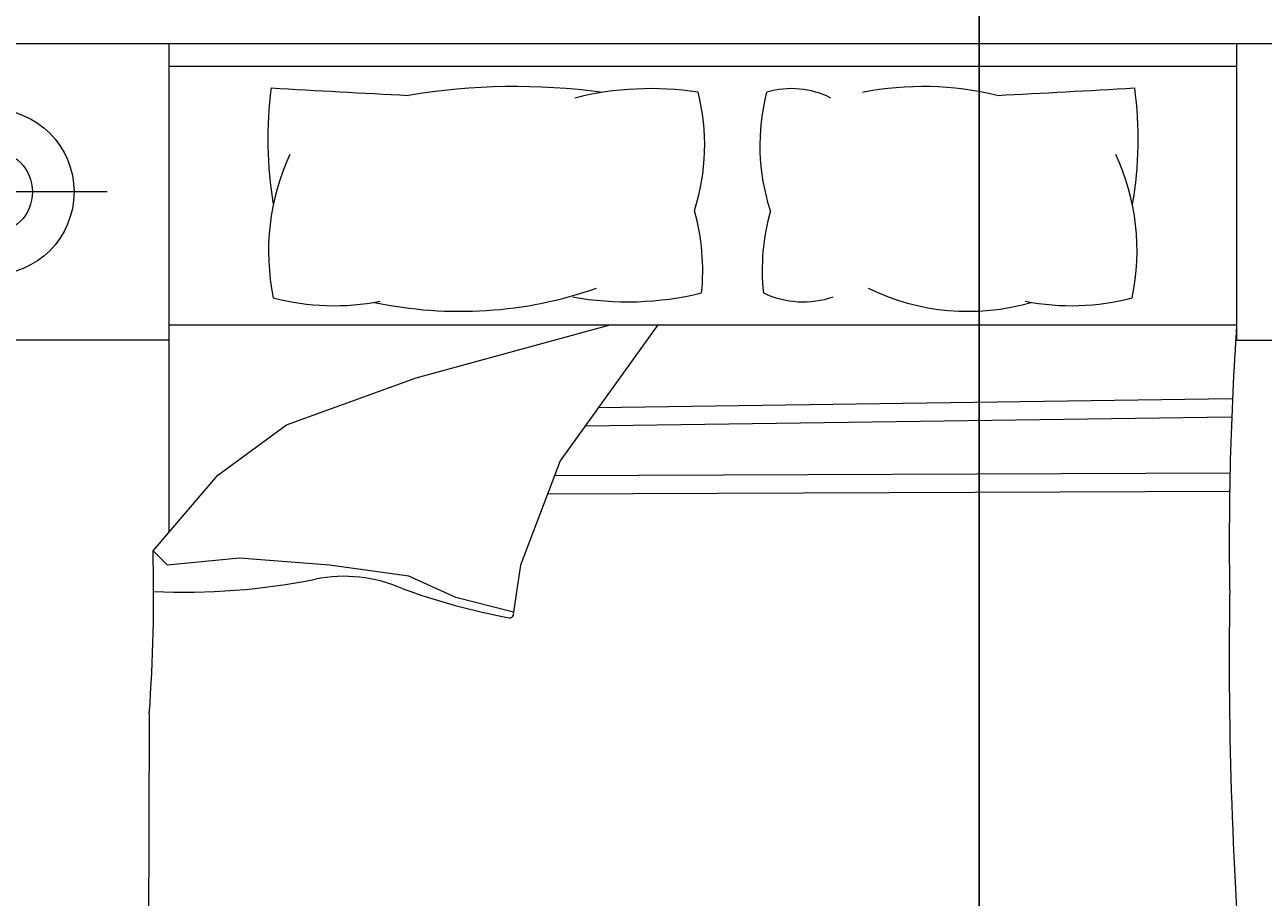
# Model space of a CAD drawing. Units: inches. Extents: x 0 to 281, y -535 to 46.
# Tile 19 of 22: x 72 to 127, y -36 to 3. Entities that reach past the tile are written whole.
import ezdxf

# ---------------------------------------------------------------- set-up
doc = ezdxf.new("R2010")
doc.units = ezdxf.units.IN
doc.header["$MEASUREMENT"] = 0
doc.layers.add('A-ANNO-DIMS', color=2, linetype='Continuous', lineweight=18)
doc.layers.add('A-FURN', color=8, linetype='Continuous', lineweight=18)
doc.styles.get("Standard").update_dxf_attribs({"font": 'arial.ttf'})
doc.dimstyles.get("Standard").update_dxf_attribs({"dimtxt": 0.18, "dimasz": 0.18, "dimexe": 0.18, "dimexo": 0.0625, "dimgap": 0.09, "dimtad": 0, "dimtih": 1, "dimtoh": 1, "dimdec": 0, "dimzin": 0, "dimdsep": 46, "dimlunit": 3, "dimtxsty": 'Standard', "dimcen": 0.09, "dimadec": 0, "dimazin": 0, "dimtfac": 1, "dimtdec": 0, "dimtofl": 0, "dimtmove": 0, "dimatfit": 3, "dimfxl": 1, "dimtolj": 1, "dimtzin": 0, "dimarcsym": 0})

# ---------------------------------------------------------------- blocks, each defined once
blk = doc.blocks.new('BEDSIDE-LAMP')
for p, q in [((5.174, 0), (5.174, 10.348)), ((0, 5.174), (10.348, 5.174))]:
    blk.add_line(p, q)
for points in [[(5.174, 5.174), (4.25, 6.774)], [(5.174, 5.174), (4.25, 3.574)]]:
    blk.add_lwpolyline(points)
for radius in [3.696, 1.848]:
    blk.add_circle((5.174, 5.174), radius)
blk = doc.blocks.new('*D45')
at = {"layer": 'A-ANNO-DIMS', "color": 0, "lineweight": -2, "transparency": 16777216}
for p, q in [((114.459, -263.348), (114.459, 46.219)), ((114.639, 46.039), (132.13, 46.039)), ((150.279, 46.039), (132.788, 46.039)), ((150.459, -263.348), (150.459, 46.219))]:
    blk.add_line(p, q, dxfattribs=at)
at = {"layer": 'A-ANNO-DIMS', "color": 0, "transparency": 16777216}
for points in [[(114.639, 46.069), (114.639, 46.009), (114.459, 46.039)], [(150.279, 46.069), (150.279, 46.009), (150.459, 46.039)]]:
    blk.add_solid(points, dxfattribs=at)
at = {"layer": 'Defpoints', "color": 0, "transparency": 16777216}
for p in [(150.459, 46.039), (114.459, -263.411), (150.459, -263.411)]:
    blk.add_point(p, dxfattribs=at)
at = {"layer": 'A-ANNO-DIMS', "color": 0, "transparency": 16777216, "insert": (132.459, 46.039), "char_height": 0.18, "attachment_point": 5}
blk.add_mtext('\\A1;3\'-0"', dxfattribs=at)
blk = doc.blocks.new('*D47')
at = {"layer": 'A-ANNO-DIMS', "color": 0, "lineweight": -2, "transparency": 16777216}
for p, q in [((114.459, -392.348), (114.459, 46.219)), ((114.639, 46.039), (132.13, 46.039)), ((150.279, 46.039), (132.788, 46.039)), ((150.459, -392.348), (150.459, 46.219))]:
    blk.add_line(p, q, dxfattribs=at)
at = {"layer": 'A-ANNO-DIMS', "color": 0, "transparency": 16777216}
for points in [[(114.639, 46.069), (114.639, 46.009), (114.459, 46.039)], [(150.279, 46.069), (150.279, 46.009), (150.459, 46.039)]]:
    blk.add_solid(points, dxfattribs=at)
at = {"layer": 'Defpoints', "color": 0, "transparency": 16777216}
for p in [(150.459, 46.039), (114.459, -392.411), (150.459, -392.411)]:
    blk.add_point(p, dxfattribs=at)
at = {"layer": 'A-ANNO-DIMS', "color": 0, "transparency": 16777216, "insert": (132.459, 46.039), "char_height": 0.18, "attachment_point": 5}
blk.add_mtext('\\A1;3\'-0"', dxfattribs=at)

msp = doc.modelspace()

# ---------------------------------------------------------------- linework, layer by layer
at = {"layer": 'A-FURN'}
for p, q in [((62.566, 1.744), (141.759, 1.744)), ((78.405, 1.744), (78.405, -19.992)), ((125.92, 0.728), (78.405, 0.728)), ((78.405, -10.77), (125.92, -10.77)), ((89.405, -13.124), (98.041, -10.77)), ((100.161, -10.77), (95.821, -16.811)), ((83.631, -15.208), (89.405, -13.124)), ((125.708, -14.06), (97.513, -14.456)), ((125.677, -14.873), (96.922, -15.279)), ((80.583, -17.452), (83.631, -15.208)), ((95.821, -16.811), (94.057, -21.46)), ((77.696, -20.818), (80.583, -17.452)), ((125.636, -17.367), (95.565, -17.486)), ((125.64, -18.18), (95.254, -18.304)), ((78.338, -21.46), (77.696, -20.818)), ((81.546, -21.139), (78.338, -21.46)), ((85.556, -21.46), (81.546, -21.139)), ((89.084, -21.941), (85.556, -21.46)), ((94.057, -21.46), (93.736, -23.544)), ((91.169, -22.902), (89.084, -21.941)), ((93.736, -23.544), (91.169, -22.902))]:
    msp.add_line(p, q, dxfattribs=at)
for points in [[(78.405, -11.454), (62.566, -11.454), (62.566, 1.744)], [(125.92, 1.744), (125.92, -11.454), (141.759, -11.454), (141.759, 1.744)]]:
    msp.add_lwpolyline(points, dxfattribs=at)
for points in [[(82.954, -0.229, 0.074897), (83.05, -5.402, -0.472817)], [(101.792, -5.691, 0.14099), (101.95, -0.414, 0.235245)], [(105.173, -5.691, -0.14099), (105.015, -0.414, -0.235245)], [(121.372, -0.229, -0.074897), (121.276, -5.402, 0.472817)], [(77.53, -28.07, 0.001242), (77.492, -43.096, -0.127202), (75.905, -50.584)]]:
    msp.add_lwpolyline(points, format="xyb", dxfattribs=at)
for centre, radius, start, end in [((126.604, 753.421), 754.913, 266.685209, 267.149775), ((93.804, -28.886), 28.721, 82.2196, 99.497), ((99.87, -14.371), 14.111, 81.5249, 103.96), ((106.102, -4.178), 3.918, 63.3437, 106.1026), ((111.973, -14.086), 13.921, 76.3427, 101.1841), ((77.721, 753.421), 754.913, 272.850225, 273.314791), ((93.043, -7.479), 10.207, 155.1316, 191.7583), ((111.283, -7.479), 10.207, 348.2417, 24.8684), ((92.456, -8.338), 9.703, 354.0129, 15.8293), ((114.509, -8.338), 9.703, 164.1707, 185.9871), ((91.365, 8.241), 18.407, 258.0397, 289.2615), ((98.817, 4.222), 13.965, 259.8617, 283.6238), ((106.631, -5.545), 4.198, 245.0183, 288.5407), ((113.967, -0.085), 10.081, 243.8761, 286.1746), ((85.778, 0.697), 10.613, 255.1039, 281.0369), ((118.547, 0.697), 10.613, 258.9631, 284.8961), ((267.887, -20.449), 142.296, 176.09997, 180.92818), ((5.085, -22.787), 72.638, 355.82941, 1.55305), ((86.195, -28.4), 6.446, 66.2616, 101.3392), ((79.051, 7.225), 29.888, 267.4519, 281.3392), ((99.234, 6.382), 30.712, 250.1194, 259.3383), ((311.205, -25.622), 185.618, 179.11454, 184.87351), ((93.556, -23.608), 0.191, 268.8623, 19.7536)]:
    msp.add_arc(centre, radius, start, end, dxfattribs=at)

# ---------------------------------------------------------------- block references
at = {"layer": 'A-FURN', "rotation": 180}
msp.add_blockref('BEDSIDE-LAMP', (75.659, 0.319), dxfattribs=at)

# ---------------------------------------------------------------- dimensions: what is measured, and where the dimension line sits
at = {"layer": 'A-ANNO-DIMS'}
for p1, p2, picture in [((114.459, -263.411), (150.459, -263.411), '*D45'), ((114.459, -392.411), (150.459, -392.411), '*D47')]:
    dim = msp.add_linear_dim(base=(150.459, 46.039), p1=p1, p2=p2, dimstyle='Standard', override={"dimdec": 1, "dimlfac": 1, "dimrnd": 0, "dimzin": 1, "dimdsep": 46, "dimlunit": 4, "dimfrac": 2}, dxfattribs=at)
    dim.commit()
    dim.dimension.update_dxf_attribs({"geometry": picture, "text_midpoint": (132.459, 46.039)})

doc.saveas('drawing.dxf')
